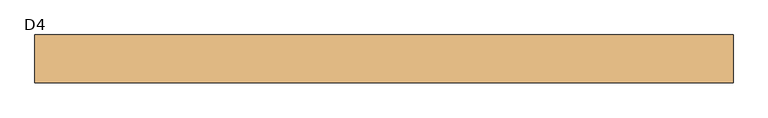
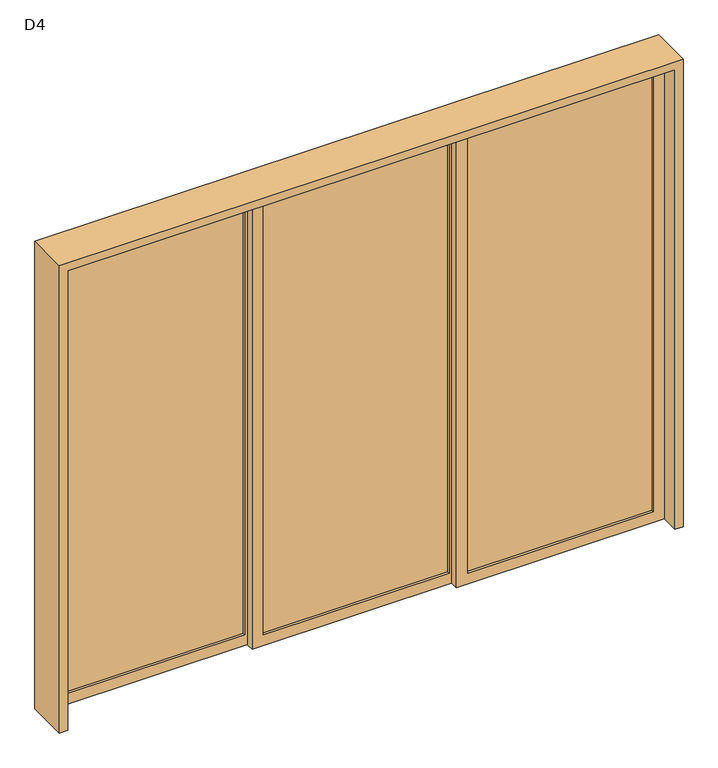
"""IFC4 building model written with IfcOpenShell, lengths in millimetres: door geometry, D4."""

from ifc_helpers import new_model, si_unit, frame, origin, place, context, project, spatial, polyline, outline, extrude, source, transform, mapped, element, save


def d4_bb962316(model_context):
    return source(origin(), model_context, "Body", "SweptSolid", [
        extrude(outline(polyline([(1530.7580012, -1.6666667), (613.2580012, -1.6666667), (613.2580012, 11.6666667), (1530.7580012, 11.6666667), (1530.7580012, -1.6666667)])), frame((0.0, 0.0, 55.0), z_axis=(0.0, 0.0, 1.0), x_axis=(1.0, 0.0, 0.0)), (0.0, 0.0, 1.0), 2290.0),
        extrude(outline(polyline([(0.0, 1585.7580012), (2400.0, 1585.7580012), (2400.0, 558.2580012), (0.0, 558.2580012), (0.0, 1585.7580012)]), holes=[polyline([(55.0, 1530.7580012), (55.0, 613.2580012), (2345.0, 613.2580012), (2345.0, 1530.7580012), (55.0, 1530.7580012)])]), frame((0.0, -15.0, 0.0), z_axis=(0.0, 1.0, 0.0), x_axis=(0.0, 0.0, 1.0)), (0.0, 0.0, 1.0), 40.0),
        extrude(outline(polyline([(544.9246679, 38.3333333), (-372.5753321, 38.3333333), (-372.5753321, 51.6666667), (544.9246679, 51.6666667), (544.9246679, 38.3333333)])), frame((0.0, 0.0, 55.0), z_axis=(0.0, 0.0, 1.0), x_axis=(1.0, 0.0, 0.0)), (0.0, 0.0, 1.0), 2290.0),
        extrude(outline(polyline([(0.0, 599.9246679), (2400.0, 599.9246679), (2400.0, -427.5753321), (0.0, -427.5753321), (0.0, 599.9246679)]), holes=[polyline([(55.0, 544.9246679), (55.0, -372.5753321), (2345.0, -372.5753321), (2345.0, 544.9246679), (55.0, 544.9246679)])]), frame((0.0, 25.0, 0.0), z_axis=(0.0, 1.0, 0.0), x_axis=(0.0, 0.0, 1.0)), (0.0, 0.0, 1.0), 40.0),
        extrude(outline(polyline([(-441.7419988, 78.3333333), (-1359.2419988, 78.3333333), (-1359.2419988, 91.6666667), (-441.7419988, 91.6666667), (-441.7419988, 78.3333333)])), frame((0.0, 0.0, 55.0), z_axis=(0.0, 0.0, 1.0), x_axis=(1.0, 0.0, 0.0)), (0.0, 0.0, 1.0), 2290.0),
        extrude(outline(polyline([(0.0, -386.7419988), (2400.0, -386.7419988), (2400.0, -1414.2419988), (0.0, -1414.2419988), (0.0, -386.7419988)]), holes=[polyline([(55.0, -441.7419988), (55.0, -1359.2419988), (2345.0, -1359.2419988), (2345.0, -441.7419988), (55.0, -441.7419988)])]), frame((0.0, 65.0, 0.0), z_axis=(0.0, 1.0, 0.0), x_axis=(0.0, 0.0, 1.0)), (0.0, 0.0, 1.0), 40.0),
        extrude(outline(polyline([(0.0, -1414.2419988), (2400.0, -1414.2419988), (2400.0, 1585.7580012), (0.0, 1585.7580012), (0.0, 1625.7580012), (2440.0, 1625.7580012), (2440.0, -1454.2419988), (0.0, -1454.2419988), (0.0, -1414.2419988)])), frame((0.0, -105.0, 0.0), z_axis=(0.0, 1.0, 0.0), x_axis=(0.0, 0.0, 1.0)), (0.0, 0.0, 1.0), 210.0),
    ])


if __name__ == "__main__":
    model = new_model("IFC4")
    model_context = context("Model", 3, world=origin())
    ifc_project = project(units=[si_unit("LENGTHUNIT", "METRE", prefix="MILLI")], contexts=[model_context])
    site = spatial("IfcSite", under=ifc_project)
    building = spatial("IfcBuilding", under=site)
    placement = place(None, origin())
    d4_shape = d4_bb962316(model_context)
    element("IfcDoor", 1, ObjectType="D4", at=placement, inside=building, context=model_context, shape_type="MappedRepresentation", body=[
        mapped(d4_shape, transform((0.0, 0.0, 0.0), x_axis=(1.0, 0.0, 0.0), y_axis=(0.0, 1.0, 0.0), z_axis=(0.0, 0.0, 1.0))),
    ])
    save(model, "model.ifc")

# Revit data of these elements
# Type "D4"
#   Type Mark = "59"
#   Operation = "UserDefined"
#   Width = 3000 mm
#   Thickness = 40 mm
#   Rough Width = 3080 mm
#   Rough Height = 2440 mm
#   Panel Width = 1027.5 mm
#   Panel Frame = 55 mm
#   Height = 2400 mm
#   Frame Depth = 40 mm
#   Glass Material = Sliding Door Glass
#   Frame Material = Sliding Door Frame
#   Function = (empty or 0)
# Element 1 (IfcDoor, "D4")
#   Materials on its faces: "Sliding Door Frame", "Sliding Door Glass"
# Materials
#   "Sliding Door Glass": colour RGB 247 247 247, transparency 0.68
#   "Sliding Door Frame": colour RGB 160 107 8, transparency 0
